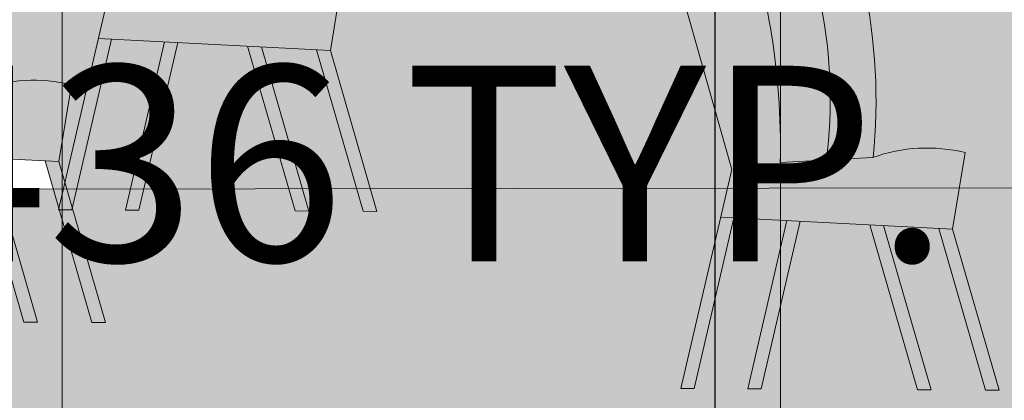
# Model space of a CAD drawing. Units: millimetres. Extents: x 11032 to 26788, y 3406 to 24505.
# Tile 7 of 78: x 15812 to 16566, y 7421 to 7713. Entities that reach past the tile are written whole.
import ezdxf

# ---------------------------------------------------------------- set-up
doc = ezdxf.new("R2010")
doc.units = ezdxf.units.MM
doc.header["$MEASUREMENT"] = 0
for name, color, linetype, lineweight in [('A-ANNO-DIMS', 2, 'Continuous', 18), ('A-FURN', 8, 'Continuous', 13), ('A-FURN-PATT', 8, 'Continuous', 13), ('A-GLAZ', 250, 'Continuous', 20), ('A-WALL-INTR', 8, 'Continuous', 18)]:
    doc.layers.add(name, color=color, linetype=linetype, lineweight=lineweight)
doc.layers.add('A-GLAZ-FRAM-PATT', color=250, linetype='Continuous', lineweight=13, true_color=0x262627)
doc.layers.add('A-WALL-INTR-PATT', color=251, linetype='Continuous', lineweight=13, true_color=0x6c6b6a)
doc.styles.get("Standard").update_dxf_attribs({"font": 'arial.ttf'})
doc.dimstyles.get("Standard").update_dxf_attribs({"dimtxt": 150, "dimasz": 100, "dimexe": 10, "dimexo": 5, "dimgap": 5, "dimtad": 0, "dimtih": 1, "dimtoh": 1, "dimdec": 0, "dimzin": 0, "dimdsep": 46, "dimtxsty": 'Standard', "dimcen": 0.09, "dimadec": 0, "dimazin": 0, "dimtfac": 1, "dimtdec": 0, "dimtofl": 0, "dimtmove": 0, "dimatfit": 3, "dimfxl": 1, "dimtolj": 1, "dimtzin": 0, "dimarcsym": 0})

# ---------------------------------------------------------------- blocks, each defined once
blk = doc.blocks.new('DINING-CHAIR-ELEV')
blk.add_line((228.68, 123.43), (51.04, 132.61))
for points in [[(0, 379.55), (49.45, 435.94), (114.12, 434.53)], [(61.18, 132.09), (30.79, 1.16), (20.53, 1.21), (59.55, 169.26), (0, 379.55), (61.9, 377.89)], [(111.9, 129.47), (82.06, 0.91), (71.8, 0.96), (101.76, 129.99)], [(165.28, 126.71), (201.76, 0.31), (212.19, 0.26), (175.85, 126.16)]]:
    blk.add_lwpolyline(points)
for points in [[(218.11, 123.98), (253.88, 0.05), (264.3, 0), (228.68, 123.43), (238.32, 182.18, 0.148451), (167.47, 178.33), (96.61, 174.48, 0.097012), (61.9, 377.89), (114.12, 434.53, -0.154833), (167.82, 178.46)], [(132.04, 176.4, 0.156877), (88.01, 406.21), (24.72, 407.74)]]:
    blk.add_lwpolyline(points, format="xyb")
blk = doc.blocks.new('*D16')
at = {"layer": 'A-ANNO-DIMS', "color": 0, "lineweight": -2, "transparency": 16777216}
for p, q in [((15741.74, 7821.05), (15812.13, 7821.05)), ((15802.13, 7721.05), (15802.13, 7685.69)), ((15802.13, 7485.11), (15802.13, 7520.47)), ((15741.74, 7385.11), (15812.13, 7385.11))]:
    blk.add_line(p, q, dxfattribs=at)
at = {"layer": 'A-ANNO-DIMS', "color": 0, "transparency": 16777216}
for points in [[(15785.47, 7721.05), (15818.8, 7721.05), (15802.13, 7821.05)], [(15785.47, 7485.11), (15818.8, 7485.11), (15802.13, 7385.11)]]:
    blk.add_solid(points, dxfattribs=at)
at = {"layer": 'Defpoints', "color": 0, "transparency": 16777216}
for p in [(15736.74, 7821.05), (15802.13, 7821.05), (15736.74, 7385.11)]:
    blk.add_point(p, dxfattribs=at)
at = {"layer": 'A-ANNO-DIMS', "color": 0, "transparency": 16777216, "insert": (15802.13, 7603.08), "char_height": 150, "attachment_point": 5}
blk.add_mtext('\\A1;CHAIR 436 TYP.', dxfattribs=at)
blk = doc.blocks.new('*D17')
at = {"layer": 'A-ANNO-DIMS', "color": 0, "lineweight": -2, "transparency": 16777216}
for p, q in [((15472.44, 7380.11), (15472.44, 7309.72)), ((15736.74, 7380.11), (15736.74, 7309.72)), ((15572.44, 7319.72), (15636.74, 7319.72)), ((15736.74, 7319.72), (15836.74, 7319.72))]:
    blk.add_line(p, q, dxfattribs=at)
at = {"layer": 'A-ANNO-DIMS', "color": 0, "transparency": 16777216}
for points in [[(15572.44, 7336.38), (15572.44, 7303.05), (15472.44, 7319.72)], [(15636.74, 7336.38), (15636.74, 7303.05), (15736.74, 7319.72)]]:
    blk.add_solid(points, dxfattribs=at)
at = {"layer": 'Defpoints', "color": 0, "transparency": 16777216}
for p in [(15472.44, 7385.11), (15736.74, 7385.11), (15736.74, 7319.72)]:
    blk.add_point(p, dxfattribs=at)
at = {"layer": 'A-ANNO-DIMS', "color": 0, "transparency": 16777216, "insert": (16266.37, 7319.72), "char_height": 150, "attachment_point": 5}
blk.add_mtext('\\A1;264 TYP.', dxfattribs=at)
blk = doc.blocks.new('*D36')
at = {"layer": 'A-ANNO-DIMS', "color": 0, "lineweight": -2, "transparency": 16777216}
for p, q in [((12301.26, 17115.89), (12301.26, 24416.86)), ((25397.4, 4466.4), (25397.4, 24416.86)), ((12401.26, 24406.86), (18569.2, 24406.86)), ((25297.4, 24406.86), (19129.47, 24406.86))]:
    blk.add_line(p, q, dxfattribs=at)
at = {"layer": 'A-ANNO-DIMS', "color": 0, "transparency": 16777216}
for points in [[(12401.26, 24423.52), (12401.26, 24390.19), (12301.26, 24406.86)], [(25297.4, 24423.52), (25297.4, 24390.19), (25397.4, 24406.86)]]:
    blk.add_solid(points, dxfattribs=at)
at = {"layer": 'Defpoints', "color": 0, "transparency": 16777216}
for p in [(25397.4, 24406.86), (12301.26, 17110.89), (25397.4, 4461.4)]:
    blk.add_point(p, dxfattribs=at)
at = {"layer": 'A-ANNO-DIMS', "color": 0, "transparency": 16777216, "insert": (18849.33, 24406.86), "char_height": 150, "attachment_point": 5}
blk.add_mtext('\\A1;13096', dxfattribs=at)
blk = doc.blocks.new('*D37')
at = {"layer": 'A-ANNO-DIMS', "color": 0, "lineweight": -2, "transparency": 16777216}
for p, q in [((18087.74, 23450.36), (11334.76, 23450.36)), ((11344.76, 23350.36), (11344.76, 14037.46)), ((11344.76, 4561.4), (11344.76, 13874.29)), ((12927.66, 4461.4), (11334.76, 4461.4))]:
    blk.add_line(p, q, dxfattribs=at)
at = {"layer": 'A-ANNO-DIMS', "color": 0, "transparency": 16777216}
for points in [[(11328.1, 23350.36), (11361.43, 23350.36), (11344.76, 23450.36)], [(11328.1, 4561.4), (11361.43, 4561.4), (11344.76, 4461.4)]]:
    blk.add_solid(points, dxfattribs=at)
at = {"layer": 'Defpoints', "color": 0, "transparency": 16777216}
for p in [(11344.76, 23450.36), (18092.74, 23450.36), (12932.66, 4461.4)]:
    blk.add_point(p, dxfattribs=at)
at = {"layer": 'A-ANNO-DIMS', "color": 0, "transparency": 16777216, "insert": (11344.76, 13955.88), "char_height": 150, "attachment_point": 5}
blk.add_mtext('\\A1;18989', dxfattribs=at)
blk = doc.blocks.new('*D49')
at = {"layer": 'A-ANNO-DIMS', "color": 0, "lineweight": -2, "transparency": 16777216}
for p, q in [((17953.45, 10206.41), (17953.45, 3494.9)), ((14996.4, 6406.4), (14996.4, 3494.9)), ((15096.4, 3504.9), (16244.67, 3504.9)), ((17853.45, 3504.9), (16705.18, 3504.9))]:
    blk.add_line(p, q, dxfattribs=at)
at = {"layer": 'A-ANNO-DIMS', "color": 0, "transparency": 16777216}
for points in [[(15096.4, 3521.57), (15096.4, 3488.23), (14996.4, 3504.9)], [(17853.45, 3521.57), (17853.45, 3488.23), (17953.45, 3504.9)]]:
    blk.add_solid(points, dxfattribs=at)
at = {"layer": 'Defpoints', "color": 0, "transparency": 16777216}
for p in [(17953.45, 10211.41), (14996.4, 6411.4), (17953.45, 3504.9)]:
    blk.add_point(p, dxfattribs=at)
at = {"layer": 'A-ANNO-DIMS', "color": 0, "transparency": 16777216, "insert": (16474.93, 3504.9), "char_height": 150, "attachment_point": 5}
blk.add_mtext('\\A1;2957', dxfattribs=at)
blk = doc.blocks.new('*D57')
at = {"layer": 'A-ANNO-DIMS', "color": 0, "lineweight": -2, "transparency": 16777216}
for p, q in [((14994.7, 7266.4), (14994.7, 24416.86)), ((20894.7, 7266.4), (20894.7, 24416.86)), ((15094.7, 24406.86), (17715.98, 24406.86)), ((20794.7, 24406.86), (18173.42, 24406.86))]:
    blk.add_line(p, q, dxfattribs=at)
at = {"layer": 'A-ANNO-DIMS', "color": 0, "transparency": 16777216}
for points in [[(15094.7, 24423.52), (15094.7, 24390.19), (14994.7, 24406.86)], [(20794.7, 24423.52), (20794.7, 24390.19), (20894.7, 24406.86)]]:
    blk.add_solid(points, dxfattribs=at)
at = {"layer": 'Defpoints', "color": 0, "transparency": 16777216}
for p in [(20894.7, 24406.86), (14994.7, 7261.4), (20894.7, 7261.4)]:
    blk.add_point(p, dxfattribs=at)
at = {"layer": 'A-ANNO-DIMS', "color": 0, "transparency": 16777216, "insert": (17944.7, 24406.86), "char_height": 150, "attachment_point": 5}
blk.add_mtext('\\A1;5900', dxfattribs=at)
blk = doc.blocks.new('*D60')
at = {"layer": 'A-ANNO-DIMS', "color": 0, "lineweight": -2, "transparency": 16777216}
for p, q in [((14994.7, 7266.4), (14994.7, 24416.86)), ((16344.7, 7266.4), (16344.7, 24416.86)), ((15094.7, 24406.86), (15448.04, 24406.86)), ((16244.7, 24406.86), (15891.36, 24406.86))]:
    blk.add_line(p, q, dxfattribs=at)
at = {"layer": 'A-ANNO-DIMS', "color": 0, "transparency": 16777216}
for points in [[(15094.7, 24423.52), (15094.7, 24390.19), (14994.7, 24406.86)], [(16244.7, 24423.52), (16244.7, 24390.19), (16344.7, 24406.86)]]:
    blk.add_solid(points, dxfattribs=at)
at = {"layer": 'Defpoints', "color": 0, "transparency": 16777216}
for p in [(16344.7, 24406.86), (14994.7, 7261.4), (16344.7, 7261.4)]:
    blk.add_point(p, dxfattribs=at)
at = {"layer": 'A-ANNO-DIMS', "color": 0, "transparency": 16777216, "insert": (15669.7, 24406.86), "char_height": 150, "attachment_point": 5}
blk.add_mtext('\\A1;1350', dxfattribs=at)
blk = doc.blocks.new('*D69')
at = {"layer": 'A-ANNO-DIMS', "color": 0, "lineweight": -2, "transparency": 16777216}
for p, q in [((13956.97, 9937.95), (14056.97, 9937.95)), ((14056.97, 9937.95), (15432.5, 8990.95)), ((17944.61, 7261.4), (17944.79, 7261.4)), ((17944.7, 7261.31), (17944.7, 7261.49))]:
    blk.add_line(p, q, dxfattribs=at)
at = {"layer": 'A-ANNO-DIMS', "color": 0, "transparency": 16777216}
blk.add_solid([(15441.95, 9004.68), (15423.05, 8977.22), (15514.87, 8934.24)], dxfattribs=at)
at = {"layer": 'Defpoints', "color": 0, "transparency": 16777216}
for p in [(15514.87, 8934.24), (17944.7, 7261.4)]:
    blk.add_point(p, dxfattribs=at)
at = {"layer": 'A-ANNO-DIMS', "color": 0, "transparency": 16777216, "insert": (13494.04, 9937.95), "char_height": 150, "attachment_point": 5}
blk.add_mtext('\\A1;2X R2950', dxfattribs=at)

msp = doc.modelspace()

# ---------------------------------------------------------------- hatches: boundary and pattern name
at = {"layer": 'A-FURN-PATT'}
h = msp.add_hatch(color=256, dxfattribs=at)
h.set_gradient(color1=(82, 15, 16), color2=(153, 0, 38), name='CURVED')
h.paths.add_polyline_path([(16952.125, 8119), (16926.017, 8147.32, 0.1568775), (16881.989, 7917.509), (16917.415, 7915.583, -0.0970121)], flags=0)
h.paths.add_polyline_path([(16899.908, 8175.64), (16964.58, 8177.046), (17014.03, 8120.657), (16954.484, 7910.365), (16972.017, 7834.84), (16977.75, 7834.965), (17027.199, 7778.576), (16967.653, 7568.284), (17006.665, 7400.238), (16996.411, 7400.187), (16966.016, 7531.114), (16925.439, 7529.018), (16955.395, 7399.983), (16945.141, 7399.932), (16915.295, 7528.494), (16861.916, 7525.736), (16825.435, 7399.337), (16815.012, 7399.285), (16851.35, 7525.19), (16809.087, 7523.007), (16773.319, 7399.078), (16762.896, 7399.026), (16798.521, 7522.461), (16788.882, 7581.207, -0.1476694), (16859.382, 7577.482, -0.1528132), (16911.41, 7830.579), (16902.125, 7870.575), (16848.746, 7867.817), (16830.506, 7804.617), (16830.506, 7793.515), (16827.302, 7793.515), (16812.265, 7741.418), (16801.842, 7741.366), (16816.893, 7793.515), (16775.261, 7793.515), (16760.15, 7741.159), (16749.727, 7741.107), (16764.853, 7793.515), (16650.704, 7793.515), (16662.994, 7750.932), (16652.571, 7750.983), (16640.296, 7793.515), (16598.663, 7793.515), (16610.879, 7751.191), (16600.455, 7751.242), (16588.255, 7793.515), (16490.425, 7793.515), (16480.749, 7751.837), (16470.495, 7751.888), (16480.159, 7793.515), (16443.833, 7793.515, -0.1094051), (16465.746, 7607.731, -0.1476694), (16536.246, 7611.456), (16526.606, 7552.71), (16562.232, 7429.275), (16551.809, 7429.327), (16516.041, 7553.255), (16473.778, 7555.439), (16510.116, 7429.534), (16499.693, 7429.586), (16463.212, 7555.985), (16409.833, 7558.743), (16379.987, 7430.181), (16369.733, 7430.232), (16394.704, 7537.793), (16394.704, 7559.524), (16359.112, 7561.363), (16328.717, 7430.435), (16318.463, 7430.486), (16344.704, 7543.521), (16344.704, 7643.635), (16302.264, 7793.515), (16205.738, 7793.515), (16227.021, 7719.773), (16216.598, 7719.825), (16195.329, 7793.515), (16153.697, 7793.515), (16174.905, 7720.032), (16164.482, 7720.084), (16143.289, 7793.515), (15844.423, 7793.515), (15844.423, 7804.617), (16140.084, 7804.617), (16128.001, 7846.483), (16191.395, 7843.208), (16201.035, 7901.954, 0.1484508), (16130.184, 7898.102), (16059.333, 7894.25, 0.0970121), (16024.622, 8097.666), (16076.839, 8154.307, -0.1548334), (16130.535, 7898.229, -0.1476694), (16201.035, 7901.954), (16191.395, 7843.208), (16202.533, 7804.617), (16299.12, 7804.617), (16297.929, 7808.825), (16347.378, 7865.214), (16412.05, 7863.808, -0.0295496), (16434.494, 7817.915), (16458.237, 7920.19), (16398.691, 8130.481), (16448.141, 8186.871), (16512.813, 8185.465, -0.1548334), (16566.508, 7929.387, -0.1476694), (16637.008, 7933.112), (16627.369, 7874.366), (16647.499, 7804.617), (16742.939, 7804.617), (16741.107, 8264.696), (17994.704, 8264.696), (17994.704, 7796.661), (18112.02, 7796.661), (18134.447, 7874.366), (18124.807, 7933.112, -0.1476694), (18195.307, 7929.387, -0.1548334), (18249.003, 8185.465), (18313.675, 8186.871), (18363.124, 8130.481), (18303.578, 7920.19), (18311.087, 7887.847, -0.0273017), (18332.016, 7930.161), (18396.688, 7931.567), (18446.137, 7875.177), (18423.905, 7796.661), (18470.25, 7796.661), (18470.25, 7785.559), (18420.761, 7785.559), (18386.591, 7664.886), (18425.604, 7496.839), (18415.35, 7496.788), (18384.955, 7627.716), (18344.377, 7625.62), (18374.333, 7496.584), (18364.079, 7496.533), (18334.233, 7625.095), (18280.854, 7622.338), (18244.373, 7495.938), (18233.95, 7495.887), (18270.288, 7621.792), (18228.026, 7619.608), (18192.257, 7495.679), (18181.834, 7495.628), (18217.46, 7619.062), (18207.82, 7677.808, -0.1476694), (18278.32, 7674.083, -0.0514181), (18278.516, 7762.821), (18273.237, 7785.559), (18171.265, 7785.559), (18161.36, 7751.242), (18150.937, 7751.191), (18160.856, 7785.559), (18119.224, 7785.559), (18109.244, 7750.983), (18098.821, 7750.932), (18108.815, 7785.559), (17852.794, 7785.559), (17866.18, 7739.181), (17855.756, 7739.233), (17842.386, 7785.559), (17800.753, 7785.559), (17814.064, 7739.44), (17803.641, 7739.492), (17790.345, 7785.559), (17694.491, 7785.559), (17685.986, 7748.922, -0.0882745), (17728.687, 7746.171), (17719.047, 7687.425), (17754.673, 7563.99), (17744.25, 7564.042), (17708.482, 7687.971), (17666.219, 7690.154), (17702.557, 7564.249), (17692.134, 7564.301), (17655.653, 7690.7), (17602.274, 7693.458), (17572.428, 7564.896), (17562.174, 7564.947), (17592.13, 7693.982), (17551.553, 7696.078), (17521.158, 7565.151), (17510.903, 7565.202), (17549.916, 7733.248), (17535.103, 7785.559), (17484.167, 7785.559), (17484.167, 7796.661), (17531.96, 7796.661), (17490.37, 7943.54), (17539.819, 7999.929), (17604.491, 7998.523, -0.0802486), (17652.289, 7869.096), (17661.422, 7908.439), (17601.876, 8118.731), (17651.326, 8175.12), (17715.998, 8173.714, -0.1548334), (17769.694, 7917.637, -0.1476694), (17840.194, 7921.361), (17830.554, 7862.615), (17849.59, 7796.661), (17894.704, 7796.661), (17894.704, 8239.696), (16741.207, 8239.696), (16742.939, 7804.617), (16768.057, 7804.617), (16785.352, 7864.542), (16775.713, 7923.288, -0.1476694), (16846.212, 7919.563, -0.1548334)], flags=17)
h.paths.add_polyline_path([(16899.908, 8175.64), (16964.58, 8177.046), (17014.03, 8120.657), (16954.484, 7910.365), (16993.496, 7742.318), (16983.242, 7742.267), (16952.847, 7873.195), (16912.27, 7871.099), (16942.225, 7742.064), (16931.971, 7742.013), (16902.125, 7870.575), (16848.746, 7867.817), (16812.265, 7741.418), (16801.842, 7741.366), (16838.181, 7867.271), (16795.918, 7865.087), (16760.15, 7741.159), (16749.727, 7741.107), (16785.352, 7864.542), (16775.713, 7923.288, -0.1476694), (16846.212, 7919.563, -0.1548334)], flags=0)
h.paths.add_polyline_path([(16899.908, 8175.64), (16964.58, 8177.046), (17014.03, 8120.657), (16954.484, 7910.365), (16972.017, 7834.84), (16977.75, 7834.965), (17027.199, 7778.576), (16967.653, 7568.284), (17006.665, 7400.238), (16996.411, 7400.187), (16966.016, 7531.114), (16925.439, 7529.018), (16955.395, 7399.983), (16945.141, 7399.932), (16915.295, 7528.494), (16861.916, 7525.736), (16825.435, 7399.337), (16815.012, 7399.285), (16851.35, 7525.19), (16809.087, 7523.007), (16773.319, 7399.078), (16762.896, 7399.026), (16798.521, 7522.461), (16788.882, 7581.207, -0.1476694), (16859.382, 7577.482, -0.1528132), (16911.41, 7830.579), (16902.125, 7870.575), (16848.746, 7867.817), (16830.506, 7804.617), (16830.506, 7793.515), (16827.302, 7793.515), (16812.265, 7741.418), (16801.842, 7741.366), (16816.893, 7793.515), (16775.261, 7793.515), (16760.15, 7741.159), (16749.727, 7741.107), (16764.853, 7793.515), (16650.704, 7793.515), (16662.994, 7750.932), (16652.571, 7750.983), (16640.296, 7793.515), (16598.663, 7793.515), (16610.879, 7751.191), (16600.455, 7751.242), (16588.255, 7793.515), (16490.425, 7793.515), (16480.749, 7751.837), (16470.495, 7751.888), (16480.159, 7793.515), (16443.833, 7793.515, -0.1094051), (16465.746, 7607.731, -0.1476694), (16536.246, 7611.456), (16526.606, 7552.71), (16562.232, 7429.275), (16551.809, 7429.327), (16516.041, 7553.255), (16473.778, 7555.439), (16510.116, 7429.534), (16499.693, 7429.586), (16463.212, 7555.985), (16409.833, 7558.743), (16379.987, 7430.181), (16369.733, 7430.232), (16394.704, 7537.793), (16394.704, 7559.524), (16359.112, 7561.363), (16328.717, 7430.435), (16318.463, 7430.486), (16344.704, 7543.521), (16344.704, 7643.635), (16302.264, 7793.515), (16205.738, 7793.515), (16227.021, 7719.773), (16216.598, 7719.825), (16195.329, 7793.515), (16153.697, 7793.515), (16174.905, 7720.032), (16164.482, 7720.084), (16143.289, 7793.515), (15844.423, 7793.515), (15844.423, 7804.617), (16140.084, 7804.617), (16128.001, 7846.483), (16191.395, 7843.208), (16201.035, 7901.954, 0.1484508), (16130.184, 7898.102), (16059.333, 7894.25, 0.0970121), (16024.622, 8097.666), (16076.839, 8154.307, -0.1548334), (16130.535, 7898.229, -0.1476694), (16201.035, 7901.954), (16191.395, 7843.208), (16202.533, 7804.617), (16299.12, 7804.617), (16297.929, 7808.825), (16347.378, 7865.214), (16412.05, 7863.808, -0.0295496), (16434.494, 7817.915), (16458.237, 7920.19), (16398.691, 8130.481), (16448.141, 8186.871), (16512.813, 8185.465, -0.1548334), (16566.508, 7929.387, -0.1476694), (16637.008, 7933.112), (16627.369, 7874.366), (16647.499, 7804.617), (16742.939, 7804.617), (16741.207, 8239.696), (16741.107, 8264.696), (17994.704, 8264.696), (17994.704, 7796.661), (18112.02, 7796.661), (18134.447, 7874.366), (18124.807, 7933.112, -0.1476694), (18195.307, 7929.387, -0.1548334), (18249.003, 8185.465), (18313.675, 8186.871), (18363.124, 8130.481), (18303.578, 7920.19), (18311.087, 7887.847, -0.0273017), (18332.016, 7930.161), (18396.688, 7931.567), (18446.137, 7875.177), (18423.905, 7796.661), (18470.25, 7796.661), (18470.25, 7785.559), (18420.761, 7785.559), (18386.591, 7664.886), (18425.604, 7496.839), (18415.35, 7496.788), (18384.955, 7627.716), (18344.377, 7625.62), (18374.333, 7496.584), (18364.079, 7496.533), (18334.233, 7625.095), (18280.854, 7622.338), (18244.373, 7495.938), (18233.95, 7495.887), (18270.288, 7621.792), (18228.026, 7619.608), (18192.257, 7495.679), (18181.834, 7495.628), (18217.46, 7619.062), (18207.82, 7677.808, -0.1476694), (18278.32, 7674.083, -0.0514181), (18278.516, 7762.821), (18273.237, 7785.559), (18171.265, 7785.559), (18161.36, 7751.242), (18150.937, 7751.191), (18160.856, 7785.559), (18119.224, 7785.559), (18109.244, 7750.983), (18098.821, 7750.932), (18108.815, 7785.559), (17852.794, 7785.559), (17866.18, 7739.181), (17855.756, 7739.233), (17842.386, 7785.559), (17800.753, 7785.559), (17814.064, 7739.44), (17803.641, 7739.492), (17790.345, 7785.559), (17694.491, 7785.559), (17685.986, 7748.922, -0.0882745), (17728.687, 7746.171), (17719.047, 7687.425), (17754.673, 7563.99), (17744.25, 7564.042), (17708.482, 7687.971), (17666.219, 7690.154), (17702.557, 7564.249), (17692.134, 7564.301), (17655.653, 7690.7), (17602.274, 7693.458), (17572.428, 7564.896), (17562.174, 7564.947), (17592.13, 7693.982), (17551.553, 7696.078), (17521.158, 7565.151), (17510.903, 7565.202), (17549.916, 7733.248), (17535.103, 7785.559), (17484.167, 7785.559), (17484.167, 7796.661), (17531.96, 7796.661), (17490.37, 7943.54), (17539.819, 7999.929), (17604.491, 7998.523, -0.0802486), (17652.289, 7869.096), (17661.422, 7908.439), (17601.876, 8118.731), (17651.326, 8175.12), (17715.998, 8173.714, -0.1548334), (17769.694, 7917.637, -0.1476694), (17840.194, 7921.361), (17830.554, 7862.615), (17849.59, 7796.661), (17894.704, 7796.661), (17894.704, 8239.696), (16741.207, 8239.696), (16742.939, 7804.617), (16768.057, 7804.617), (16785.352, 7864.542), (16775.713, 7923.288, -0.1476694), (16846.212, 7919.563, -0.1548334)], flags=17)
h = msp.add_hatch(color=256, dxfattribs=at)
h.set_gradient(color1=(153, 27, 30), color2=(153, 38, 0), name='SPHERICAL')
h.paths.add_polyline_path([(15534.344, 7763), (15472.44, 7764.657), (15531.986, 7554.365), (15523.479, 7517.719), (15640.736, 7511.661), (15653.713, 7567.556, 0.0295203), (15639.906, 7563.436), (15569.055, 7559.583, 0.0970121)], flags=16)
h.paths.add_polyline_path([(15560.453, 7791.32), (15534.344, 7763, -0.0970121), (15569.055, 7559.583), (15604.48, 7561.509, 0.1568775)], flags=16)
h.paths.add_polyline_path([(15586.562, 7819.64), (15560.453, 7791.32, -0.1568775), (15604.48, 7561.509), (15640.246, 7563.454, 0.154898)], flags=17)
h.paths.add_polyline_path([(15560.453, 7791.32), (15497.165, 7792.851), (15472.44, 7764.657), (15534.344, 7763)], flags=16)
h.paths.add_polyline_path([(15586.562, 7819.64), (15521.889, 7821.046), (15497.165, 7792.851), (15560.453, 7791.32)], flags=17)
h.paths.add_polyline_path([(15790.874, 7662.689, 0.021469), (15780.879, 7659.53), (15710.028, 7655.677, 0.0970121), (15675.317, 7859.094), (15665.772, 7859.35), (15665.799, 7675.745), (15672.959, 7650.459), (15665.807, 7619.654), (15665.808, 7613.744), (15790.755, 7607.288)], flags=17)
h.paths.add_polyline_path([(15665.772, 7859.35), (15613.413, 7860.751), (15665.799, 7675.745)], flags=16)
h.paths.add_polyline_path([(15701.426, 7887.414), (15665.767, 7888.277), (15665.772, 7859.35), (15675.317, 7859.094)], flags=16)
h.paths.add_polyline_path([(15727.534, 7915.735), (15665.763, 7917.077), (15665.767, 7888.277), (15701.426, 7887.414)], flags=17)
h.paths.add_polyline_path([(15665.763, 7917.077), (15662.862, 7917.14), (15638.137, 7888.946), (15665.767, 7888.277)], flags=17)
h.paths.add_polyline_path([(15665.767, 7888.277), (15638.137, 7888.946), (15613.413, 7860.751), (15665.772, 7859.35)], flags=16)
h.paths.add_polyline_path([(15701.426, 7887.414), (15675.317, 7859.094, -0.0970121), (15710.028, 7655.677), (15745.453, 7657.604, 0.1568775)], flags=16)
h.paths.add_polyline_path([(15844.495, 7664.925), (15844.384, 7864.461), (15821.312, 7945.94), (15870.762, 8002.329), (15935.434, 8000.923, -0.1195917), (15991.005, 7804.617), (16002.667, 7804.617), (16022.264, 7889.032), (15962.718, 8099.323), (16024.622, 8097.666), (16076.839, 8154.307, -0.1548334), (16130.535, 7898.229, -0.1476694), (16201.035, 7901.954), (16191.395, 7843.208), (16202.533, 7804.617), (16299.12, 7804.617), (16297.929, 7808.825), (16347.378, 7865.214), (16412.05, 7863.808, -0.0295496), (16434.494, 7817.915), (16458.237, 7920.19), (16398.691, 8130.481), (16460.595, 8128.825), (16512.813, 8185.465, -0.1548334), (16566.508, 7929.387, -0.1476694), (16637.008, 7933.112), (16627.369, 7874.366), (16647.499, 7804.617), (16830.506, 7804.617), (16830.506, 7793.515), (16650.704, 7793.515), (16662.994, 7750.932), (16652.571, 7750.983), (16640.296, 7793.515), (16490.425, 7793.515), (16480.749, 7751.837), (16470.495, 7751.888), (16480.159, 7793.515), (16443.833, 7793.515, -0.1094051), (16465.746, 7607.731, -0.1476694), (16536.246, 7611.456), (16526.606, 7552.71), (16562.232, 7429.275), (16551.809, 7429.327), (16516.041, 7553.255), (16473.778, 7555.439), (16510.116, 7429.534), (16499.693, 7429.586), (16463.212, 7555.985), (16409.833, 7558.743), (16379.987, 7430.181), (16369.733, 7430.232), (16394.704, 7537.793), (16394.704, 7559.524), (16359.112, 7561.363), (16328.717, 7430.435), (16318.463, 7430.486), (16344.704, 7543.521), (16344.704, 7643.635), (16302.264, 7793.515), (16205.738, 7793.515), (16227.021, 7719.773), (16216.598, 7719.825), (16195.329, 7793.515), (16153.697, 7793.515), (16174.905, 7720.032), (16164.482, 7720.084), (16143.289, 7793.515), (16061.685, 7793.515), (16051.641, 7750.248, -0.0167144), (16059.629, 7748.571), (16049.99, 7689.825), (16085.615, 7566.39), (16075.192, 7566.442), (16039.424, 7690.371), (15997.161, 7692.554), (16033.5, 7566.649), (16023.077, 7566.701), (15986.595, 7693.1), (15933.216, 7695.858), (15903.371, 7567.296), (15893.116, 7567.347), (15923.072, 7696.382), (15882.495, 7698.478), (15852.409, 7568.882), (15877.716, 7481.201), (15867.293, 7481.253), (15842.372, 7567.599), (15841.846, 7567.602), (15842.08, 7568.609), (15831.524, 7605.182), (15790.755, 7607.288), (15790.744, 7602.228), (15825.6, 7481.46), (15815.177, 7481.512), (15778.696, 7607.911), (15725.317, 7610.669), (15701.389, 7507.6), (15736.743, 7385.107), (15726.32, 7385.159), (15696.749, 7487.614), (15695.471, 7482.107), (15685.217, 7482.158), (15691.06, 7507.327), (15690.552, 7509.088), (15650.881, 7511.137), (15649.743, 7506.234), (15684.627, 7385.366), (15674.204, 7385.418), (15645.103, 7486.248), (15644.2, 7482.362), (15633.946, 7482.413), (15639.413, 7505.961), (15637.723, 7511.817), (15584.344, 7514.575), (15554.498, 7386.013), (15544.244, 7386.064), (15574.2, 7515.099), (15533.623, 7517.195), (15503.228, 7386.268), (15492.974, 7386.319), (15531.986, 7554.365), (15472.44, 7764.657), (15497.165, 7792.851), (15521.889, 7821.046), (15586.562, 7819.64, -0.1548334), (15640.257, 7563.563, -0.0287549), (15653.713, 7567.556), (15665.807, 7619.654), (15665.799, 7675.745), (15613.413, 7860.751), (15638.137, 7888.946), (15662.862, 7917.14), (15665.763, 7917.077), (15727.534, 7915.735, -0.1548334), (15781.23, 7659.657, -0.1322263)])
h = msp.add_hatch(color=256, dxfattribs=at)
h.set_gradient(color1=(153, 27, 30), color2=(153, 38, 0), name='SPHERICAL')
h.paths.add_polyline_path([(15710.028, 7655.677), (15745.453, 7657.604, 0.1568775), (15701.426, 7887.414), (15675.317, 7859.094, -0.0970121)], flags=16)
h.paths.add_polyline_path([(15790.755, 7607.288), (15790.874, 7662.689, 0.021469), (15780.879, 7659.53), (15710.028, 7655.677, 0.0970121), (15675.317, 7859.094), (15665.772, 7859.35), (15665.799, 7675.745), (15672.959, 7650.459), (15665.807, 7619.654), (15665.808, 7613.744)], flags=17)
h.paths.add_polyline_path([(15653.713, 7567.556), (15665.807, 7619.654), (15665.799, 7675.745), (15613.413, 7860.751), (15662.862, 7917.14), (15727.534, 7915.735, -0.1548334), (15781.23, 7659.657, -0.1322263), (15844.495, 7664.925), (15844.384, 7864.461), (15821.312, 7945.94), (15883.216, 7944.283), (15935.434, 8000.923, -0.1195917), (15991.005, 7804.617), (16002.667, 7804.617), (16022.264, 7889.032), (15962.718, 8099.323), (16024.622, 8097.666), (16076.839, 8154.307, -0.1548334), (16130.535, 7898.229, -0.1476694), (16201.035, 7901.954), (16191.395, 7843.208), (16202.533, 7804.617), (16830.506, 7804.617), (16830.506, 7793.515), (16205.738, 7793.515), (16227.021, 7719.773), (16216.598, 7719.825), (16195.329, 7793.515), (16153.697, 7793.515), (16174.905, 7720.032), (16164.482, 7720.084), (16143.289, 7793.515), (16061.685, 7793.515), (16051.641, 7750.248, -0.0167144), (16059.629, 7748.571), (16049.99, 7689.825), (16085.615, 7566.39), (16075.192, 7566.442), (16039.424, 7690.371), (15997.161, 7692.554), (16033.5, 7566.649), (16023.077, 7566.701), (15986.595, 7693.1), (15933.216, 7695.858), (15903.371, 7567.296), (15893.116, 7567.347), (15923.072, 7696.382), (15882.495, 7698.478), (15852.409, 7568.882), (15877.716, 7481.201), (15867.293, 7481.253), (15842.372, 7567.599), (15841.846, 7567.602), (15842.08, 7568.609), (15831.524, 7605.182), (15790.755, 7607.288), (15790.744, 7602.228), (15825.6, 7481.46), (15815.177, 7481.512), (15778.696, 7607.911), (15725.317, 7610.669), (15701.389, 7507.6), (15736.743, 7385.107), (15726.32, 7385.159), (15696.749, 7487.614), (15695.471, 7482.107), (15685.217, 7482.158), (15705.262, 7568.502, 0.0841685), (15664.448, 7569.579), (15644.2, 7482.362), (15633.946, 7482.413), (15653.713, 7567.556, 0.0295203), (15639.906, 7563.436), (15569.055, 7559.583, 0.0970121), (15534.344, 7763), (15472.44, 7764.657), (15521.889, 7821.046), (15586.562, 7819.64, -0.1548334), (15640.257, 7563.563, -0.0287549)])
at = {"layer": 'A-GLAZ-FRAM-PATT'}
h = msp.add_hatch(color=256, dxfattribs=at)
h.paths.add_polyline_path([(17944.704, 7311.399), (16344.704, 7311.399), (16344.704, 7261.399), (17944.704, 7261.399)], flags=17)
h.paths.add_polyline_path([(16344.704, 7311.399), (15045.135, 7311.399, -0.9829047), (20844.273, 7311.399), (19544.704, 7311.399), (19544.704, 7261.399), (20894.704, 7261.399, 0.5148441), (16985.951, 10051.255, 0.3202679), (14994.704, 7261.399), (16344.704, 7261.399)])
h.paths.add_polyline_path([(18744.704, 7311.399), (17944.704, 7311.399), (17944.704, 7261.399), (18744.704, 7261.399)], flags=17)
h.paths.add_polyline_path([(19544.704, 7311.399), (18744.704, 7311.399), (18744.704, 7261.399), (19544.704, 7261.399)], flags=17)
h.paths.add_polyline_path([(18694.704, 7361.399), (17994.704, 7361.399), (17994.704, 7311.399), (18694.704, 7311.399)], flags=17)
h.paths.add_polyline_path([(18744.704, 7361.399), (18694.704, 7361.399), (18694.704, 7311.399), (18744.704, 7311.399)], flags=17)
h.paths.add_polyline_path([(17194.704, 7361.399), (17144.704, 7361.399), (17144.704, 7311.399), (17194.704, 7311.399)], flags=17)
h.paths.add_polyline_path([(17431.432, 7361.399), (17194.704, 7361.399), (17194.704, 7311.399), (17431.699, 7311.399)], flags=17)
h.paths.add_polyline_path([(17894.704, 7361.399), (17431.432, 7361.399), (17431.699, 7311.399), (17894.704, 7311.399)], flags=17)
h.paths.add_polyline_path([(17944.704, 7361.399), (17894.704, 7361.399), (17894.704, 7311.399), (17944.704, 7311.399)], flags=17)
h.paths.add_polyline_path([(17994.704, 7361.399), (17944.704, 7361.399), (17944.704, 7311.399), (17994.704, 7311.399)], flags=17)
h = msp.add_hatch(color=256, dxfattribs=at)
h.paths.add_polyline_path([(16734.609, 9896.863, 0.0333754), (16394.704, 9712.419), (16394.704, 7804.617), (16431.407, 7804.617), (16458.237, 7920.19), (16398.691, 8130.481), (16448.141, 8186.871), (16512.813, 8185.465, -0.1548334), (16566.508, 7929.387, -0.1476694), (16637.008, 7933.112), (16627.369, 7874.366), (16647.499, 7804.617), (16742.939, 7804.617)])
h.paths.add_polyline_path([(17094.704, 9961.399), (16886.403, 9961.399, 0.0142221), (16734.609, 9896.863), (16741.107, 8264.696), (17094.704, 8264.696)])
h.paths.add_polyline_path([(17417.202, 10027.292), (17194.704, 10011.399), (17194.704, 8264.696), (17426.61, 8264.696)])
h.paths.add_polyline_path([(17144.704, 8239.696), (17094.704, 8239.696), (17094.704, 7361.399), (16394.704, 7361.399), (16394.704, 7493.572), (16379.987, 7430.181), (16369.733, 7430.232), (16394.704, 7537.793), (16394.704, 7559.524), (16359.112, 7561.363), (16344.704, 7499.3), (16344.704, 7311.399), (17144.704, 7311.399)])
h.paths.add_polyline_path([(17194.704, 8239.696), (17144.704, 8239.696), (17144.704, 7361.399), (17194.704, 7361.399)])
at = {"layer": 'A-WALL-INTR-PATT'}
msp.add_hatch(color=256, dxfattribs=at).paths.add_polyline_path([(15843.607, 9260.247, 0.0062633), (15794.195, 9206.987), (15790.874, 7662.689, -0.1112179), (15844.495, 7664.925), (15844.384, 7864.461), (15821.312, 7945.94), (15844.324, 7972.181)])
h = msp.add_hatch(color=256, dxfattribs=at)
h.paths.add_polyline_path([(15302.659, 8457.059, 0.0281002), (15185.248, 8153.253), (15233.282, 7717.599), (15314.374, 7311.399), (15467.334, 7311.399), (15381.661, 7740.545)])
h.paths.add_polyline_path([(16344.704, 7543.521), (16344.704, 7643.635), (16302.264, 7793.515), (16205.738, 7793.515), (16227.021, 7719.773), (16216.598, 7719.825), (16195.329, 7793.515), (16153.697, 7793.515), (16174.905, 7720.032), (16164.482, 7720.084), (16143.289, 7793.515), (16061.685, 7793.515), (16051.641, 7750.248, -0.0167144), (16059.629, 7748.571), (16049.99, 7689.825), (16085.615, 7566.39), (16075.192, 7566.442), (16039.424, 7690.371), (15997.161, 7692.554), (16033.5, 7566.649), (16023.077, 7566.701), (15986.595, 7693.1), (15933.216, 7695.858), (15903.371, 7567.296), (15893.116, 7567.347), (15923.072, 7696.382), (15882.495, 7698.478), (15852.409, 7568.882), (15877.716, 7481.201), (15867.293, 7481.253), (15844.553, 7560.041), (15844.691, 7311.399), (16344.704, 7311.399), (16344.704, 7499.3), (16328.717, 7430.435), (16318.463, 7430.486)])
h.paths.add_polyline_path([(16742.983, 7793.515), (16650.704, 7793.515), (16662.994, 7750.932), (16652.571, 7750.983), (16640.296, 7793.515), (16598.663, 7793.515), (16610.879, 7751.191), (16600.455, 7751.242), (16588.255, 7793.515), (16490.425, 7793.515), (16480.749, 7751.837), (16470.495, 7751.888), (16480.159, 7793.515), (16443.833, 7793.515, -0.1094051), (16465.746, 7607.731, -0.1476694), (16536.246, 7611.456), (16526.606, 7552.71), (16562.232, 7429.275), (16551.809, 7429.327), (16516.041, 7553.255), (16473.778, 7555.439), (16510.116, 7429.534), (16499.693, 7429.586), (16463.212, 7555.985), (16409.833, 7558.743), (16394.704, 7493.572), (16394.704, 7361.399), (16744.704, 7361.399)])
h.paths.add_polyline_path([(17094.704, 8239.696), (16741.207, 8239.696), (16742.939, 7804.617), (16768.057, 7804.617), (16785.352, 7864.542), (16775.713, 7923.288, -0.1476694), (16846.212, 7919.563, -0.1548334), (16899.908, 8175.64), (16964.58, 8177.046), (17014.03, 8120.657), (16954.484, 7910.365), (16972.017, 7834.84), (16977.75, 7834.965), (17027.199, 7778.576), (16967.653, 7568.284), (17006.665, 7400.238), (16996.411, 7400.187), (16966.016, 7531.114), (16925.439, 7529.018), (16955.395, 7399.983), (16945.141, 7399.932), (16915.295, 7528.494), (16861.916, 7525.736), (16825.435, 7399.337), (16815.012, 7399.285), (16851.35, 7525.19), (16809.087, 7523.007), (16773.319, 7399.078), (16762.896, 7399.026), (16798.521, 7522.461), (16788.882, 7581.207, -0.1476694), (16859.382, 7577.482, -0.1528132), (16911.41, 7830.579), (16902.125, 7870.575), (16848.746, 7867.817), (16830.506, 7804.617), (16830.506, 7793.515), (16827.302, 7793.515), (16812.265, 7741.418), (16801.842, 7741.366), (16816.893, 7793.515), (16775.261, 7793.515), (16760.15, 7741.159), (16749.727, 7741.107), (16764.853, 7793.515), (16742.983, 7793.515), (16744.704, 7361.399), (17094.704, 7361.399)])
h.paths.add_polyline_path([(18950.929, 7931.023), (19015.601, 7932.429), (19065.05, 7876.04), (19005.504, 7665.748), (19014.012, 7629.102, -0.129191), (19069.892, 7841.762), (19134.564, 7843.167), (19168.958, 7803.946), (19202.145, 7841.791), (19246.92, 7840.817), (19212.932, 7960.847), (19262.382, 8017.236), (19327.054, 8015.831, -0.134919), (19382.824, 7793.43), (19562.845, 7793.43, -0.1257757), (19618.686, 8000.275), (19683.358, 8001.68), (19732.808, 7945.291), (19689.807, 7793.43), (19753.644, 7793.43, -0.0966843), (19805.964, 7950.707), (19870.637, 7952.112), (19920.086, 7895.723), (19891.121, 7793.43), (20039.255, 7793.43, -0.0897865), (20089.9, 7938.993), (20154.572, 7940.399), (20204.021, 7884.01), (20144.475, 7673.718), (20152.983, 7637.072, -0.1476694), (20223.483, 7633.347, -0.1548334), (20277.178, 7889.425), (20341.85, 7890.831), (20391.3, 7834.441), (20331.754, 7624.15), (20370.766, 7456.103), (20360.512, 7456.052), (20330.117, 7586.98), (20289.54, 7584.884), (20319.496, 7455.848), (20309.241, 7455.797), (20279.396, 7584.359), (20226.017, 7581.602), (20189.536, 7455.202), (20179.112, 7455.151), (20215.451, 7581.056), (20173.188, 7578.872), (20169.478, 7566.018), (20183.488, 7505.671), (20173.234, 7505.62), (20163.789, 7546.305), (20137.42, 7454.943), (20126.997, 7454.892), (20159.149, 7566.291), (20142.839, 7636.548), (20102.261, 7634.452), (20132.217, 7505.417), (20121.963, 7505.366), (20092.117, 7633.928), (20038.738, 7631.17), (20002.257, 7504.771), (19991.834, 7504.719), (20028.172, 7630.624), (19985.91, 7628.44), (19950.141, 7504.512), (19939.718, 7504.46), (19975.344, 7627.895), (19965.704, 7686.641, -0.1476694), (20036.204, 7682.916, -0.0576487), (20037.659, 7782.328), (19887.977, 7782.328), (19860.54, 7685.431), (19899.552, 7517.385), (19889.298, 7517.334), (19858.903, 7648.261), (19818.326, 7646.165), (19848.282, 7517.13), (19838.028, 7517.079), (19808.182, 7645.641), (19754.803, 7642.883), (19718.322, 7516.484), (19707.899, 7516.432), (19744.237, 7642.337), (19701.974, 7640.154), (19698.264, 7627.3), (19712.274, 7566.953), (19702.02, 7566.902), (19692.575, 7607.587), (19666.206, 7516.225), (19655.783, 7516.173), (19687.935, 7627.573), (19671.625, 7697.83), (19631.048, 7695.733), (19661.003, 7566.698), (19650.749, 7566.647), (19620.903, 7695.209), (19567.524, 7692.451), (19531.043, 7566.052), (19520.62, 7566), (19556.959, 7691.905), (19514.696, 7689.722), (19478.928, 7565.793), (19468.505, 7565.741), (19473, 7581.318), (19466.812, 7581.349), (19431.044, 7705.278), (19388.781, 7707.461), (19425.12, 7581.556), (19414.696, 7581.608), (19378.215, 7708.007), (19324.836, 7710.765), (19318.877, 7685.094, -0.0584523), (19320.513, 7584.307, -0.1476694), (19391.013, 7588.032), (19381.373, 7529.286), (19416.999, 7405.852), (19406.576, 7405.903), (19370.808, 7529.832), (19328.545, 7532.016), (19364.883, 7406.111), (19354.46, 7406.162), (19317.979, 7532.562), (19264.6, 7535.319), (19234.754, 7406.757), (19224.5, 7406.808), (19254.456, 7535.844), (19213.879, 7537.94), (19183.484, 7407.012), (19173.23, 7407.063), (19212.242, 7575.11), (19168.16, 7730.789), (19124.467, 7576.487), (19163.48, 7408.44), (19153.225, 7408.389), (19122.83, 7539.317), (19082.253, 7537.22), (19112.209, 7408.185), (19101.955, 7408.134), (19072.109, 7536.696), (19035.898, 7534.825), (19044.517, 7497.701), (19034.262, 7497.65), (19025.754, 7534.301), (19018.73, 7533.938), (18982.249, 7407.539), (18971.826, 7407.487), (19008.164, 7533.392), (18985.177, 7532.205), (18993.246, 7497.447), (18982.992, 7497.396), (18975.033, 7531.681), (18965.902, 7531.209), (18930.133, 7407.28), (18919.71, 7407.228), (18955.336, 7530.663), (18945.696, 7589.409, -0.0318483), (18960.996, 7592.142), (18953.146, 7625.958), (18899.767, 7623.2), (18863.286, 7496.801), (18852.863, 7496.749), (18889.201, 7622.654), (18846.938, 7620.47), (18811.17, 7496.542), (18800.747, 7496.49), (18836.373, 7619.924), (18826.733, 7678.67, -0.1476694), (18897.233, 7674.946, -0.1548334)], flags=16)
h = msp.add_hatch(color=256, dxfattribs=at)
h.set_gradient(color1=(254, 234, 185), color2=(254, 204, 102), name='CURVED')
h.paths.add_polyline_path([(15260.167, 7582.928), (15062.56, 7582.722, 0.023451), (15045.135, 7311.399), (15314.374, 7311.399)])
h.paths.add_polyline_path([(15413.095, 7583.087), (15260.167, 7582.928), (15314.374, 7311.399), (15467.334, 7311.399)])
h.paths.add_polyline_path([(15531.986, 7554.365), (15523.82, 7583.203), (15413.095, 7583.087), (15467.334, 7311.399), (15790.119, 7311.399), (15790.667, 7566.433), (15785.748, 7583.476), (15718.988, 7583.406), (15701.389, 7507.6), (15736.743, 7385.107), (15726.32, 7385.159), (15696.749, 7487.614), (15695.471, 7482.107), (15685.217, 7482.158), (15691.06, 7507.327), (15690.552, 7509.088), (15650.881, 7511.137), (15649.743, 7506.234), (15684.627, 7385.366), (15674.204, 7385.418), (15646.227, 7482.352), (15633.946, 7482.413), (15639.413, 7505.961), (15637.723, 7511.817), (15584.344, 7514.575), (15554.498, 7386.013), (15544.244, 7386.064), (15574.2, 7515.099), (15533.623, 7517.195), (15503.228, 7386.268), (15492.974, 7386.319)])
h.paths.add_polyline_path([(16344.704, 7499.3), (16328.717, 7430.435), (16318.463, 7430.486), (16344.704, 7543.521), (16344.704, 7584.059), (16080.595, 7583.783), (16085.615, 7566.39), (16075.192, 7566.442), (16070.19, 7583.773), (16028.57, 7583.729), (16033.5, 7566.649), (16023.077, 7566.701), (16018.165, 7583.718), (15907.156, 7583.603), (15903.371, 7567.296), (15893.116, 7567.347), (15896.888, 7583.592), (15855.814, 7583.549), (15852.409, 7568.882), (15877.716, 7481.201), (15867.293, 7481.253), (15844.553, 7560.041), (15844.691, 7311.399), (16344.704, 7311.399)])
h.paths.add_polyline_path([(15844.553, 7560.041), (15842.372, 7567.599), (15841.846, 7567.602), (15842.08, 7568.609), (15837.773, 7583.53), (15796.153, 7583.487), (15825.6, 7481.46), (15815.177, 7481.512), (15790.667, 7566.433), (15790.119, 7311.399), (15844.691, 7311.399)])
h.paths.add_polyline_path([(16394.704, 7493.572), (16379.987, 7430.181), (16369.733, 7430.232), (16394.704, 7537.793), (16394.704, 7559.524), (16359.112, 7561.363), (16344.704, 7499.3), (16344.704, 7311.399), (17144.704, 7311.399), (17144.704, 7584.893), (17094.704, 7584.841), (17094.704, 7361.399), (16394.704, 7361.399)])
h.paths.add_polyline_path([(17430.237, 7585.191), (17194.704, 7584.945), (17194.704, 7361.399), (17431.432, 7361.399)])
h.paths.add_polyline_path([(17894.704, 7585.675), (17748.458, 7585.522), (17754.673, 7563.99), (17744.25, 7564.042), (17738.053, 7585.511), (17696.433, 7585.468), (17702.557, 7564.249), (17692.134, 7564.301), (17686.028, 7585.457), (17577.175, 7585.344), (17572.428, 7564.896), (17562.174, 7564.947), (17566.907, 7585.333), (17525.833, 7585.29), (17521.158, 7565.151), (17510.903, 7565.202), (17515.565, 7585.28), (17430.237, 7585.191), (17431.432, 7361.399), (17894.704, 7361.399)])
h.paths.add_polyline_path([(18694.704, 7586.509), (18404.857, 7586.207), (18425.604, 7496.839), (18415.35, 7496.788), (18394.593, 7586.196), (18353.54, 7586.153), (18374.333, 7496.584), (18364.079, 7496.533), (18343.276, 7586.142), (18270.386, 7586.066), (18244.373, 7495.938), (18233.95, 7495.887), (18259.974, 7586.056), (18218.329, 7586.012), (18192.257, 7495.679), (18181.834, 7495.628), (18207.918, 7586.001), (17994.704, 7585.779), (17994.704, 7361.399), (18694.704, 7361.399)])
h.paths.add_polyline_path([(19317.979, 7532.562), (19264.6, 7535.319), (19234.754, 7406.757), (19224.5, 7406.808), (19254.456, 7535.844), (19213.879, 7537.94), (19183.484, 7407.012), (19173.23, 7407.063), (19212.242, 7575.11), (19208.862, 7587.045), (19127.433, 7586.96), (19124.467, 7576.487), (19163.48, 7408.44), (19153.225, 7408.389), (19122.83, 7539.317), (19082.253, 7537.22), (19112.209, 7408.185), (19101.955, 7408.134), (19072.109, 7536.696), (19035.898, 7534.825), (19044.517, 7497.701), (19034.262, 7497.65), (19025.754, 7534.301), (19018.73, 7533.938), (18982.249, 7407.539), (18971.826, 7407.487), (19008.164, 7533.392), (18985.177, 7532.205), (18993.246, 7497.447), (18982.992, 7497.396), (18975.033, 7531.681), (18965.902, 7531.209), (18930.133, 7407.28), (18919.71, 7407.228), (18955.336, 7530.663), (18946.129, 7586.771), (18889.236, 7586.712), (18863.286, 7496.801), (18852.863, 7496.749), (18878.825, 7586.701), (18837.179, 7586.657), (18811.17, 7496.542), (18800.747, 7496.49), (18826.768, 7586.647), (18794.704, 7586.613), (18794.704, 7361.399), (19494.704, 7361.399), (19494.704, 7587.343), (19485.145, 7587.333), (19478.928, 7565.793), (19468.505, 7565.741), (19473, 7581.318), (19466.812, 7581.349), (19465.091, 7587.312), (19423.471, 7587.269), (19425.12, 7581.556), (19414.696, 7581.608), (19413.066, 7587.258), (19390.882, 7587.235), (19381.373, 7529.286), (19416.999, 7405.852), (19406.576, 7405.903), (19370.808, 7529.832), (19328.545, 7532.016), (19364.883, 7406.111), (19354.46, 7406.162)])
h.paths.add_polyline_path([(19990.261, 7587.86), (19974.192, 7587.843), (19950.141, 7504.512), (19939.718, 7504.46), (19963.781, 7587.832), (19883.217, 7587.748), (19899.552, 7517.385), (19889.298, 7517.334), (19872.954, 7587.737), (19831.9, 7587.695), (19848.282, 7517.13), (19838.028, 7517.079), (19821.637, 7587.684), (19738.846, 7587.598), (19718.322, 7516.484), (19707.899, 7516.432), (19728.435, 7587.587), (19707.489, 7587.565), (19712.274, 7566.953), (19702.02, 7566.902), (19697.225, 7587.554), (19686.79, 7587.543), (19666.206, 7516.225), (19655.783, 7516.173), (19676.379, 7587.532), (19656.172, 7587.511), (19661.003, 7566.698), (19650.749, 7566.647), (19645.908, 7587.501), (19544.704, 7587.395), (19544.704, 7311.399), (19990.261, 7311.399)])
h.paths.add_polyline_path([(20190.261, 7455.206), (20179.112, 7455.151), (20190.261, 7493.779), (20190.261, 7579.754), (20173.188, 7578.872), (20169.478, 7566.018), (20183.488, 7505.671), (20173.234, 7505.62), (20163.789, 7546.305), (20137.42, 7454.943), (20126.997, 7454.892), (20159.149, 7566.291), (20154.102, 7588.03), (20113.048, 7587.988), (20132.217, 7505.417), (20121.963, 7505.366), (20102.785, 7587.977), (20026.249, 7587.897), (20002.257, 7504.771), (19990.261, 7504.711), (19990.261, 7311.399), (20190.261, 7311.399)])
h.paths.add_polyline_path([(20340.261, 7543.283), (20330.117, 7586.98), (20289.54, 7584.884), (20319.496, 7455.848), (20309.241, 7455.797), (20279.396, 7584.359), (20226.017, 7581.602), (20190.261, 7457.717), (20190.261, 7311.399), (20340.261, 7311.399)])
h.paths.add_polyline_path([(20826.171, 7588.731), (20340.261, 7588.225), (20340.261, 7587.504), (20370.766, 7456.103), (20360.512, 7456.052), (20340.261, 7543.283), (20340.261, 7311.399), (20844.273, 7311.399, 0.0239726)])

# ---------------------------------------------------------------- linework, layer by layer
at = {"layer": 'A-GLAZ'}
for p, q in [((16394.704, 7361.399), (16394.704, 9712.419)), ((16344.704, 7261.399), (16344.704, 9680.076))]:
    msp.add_line(p, q, dxfattribs=at)
for radius, start, end in [(2900, 0.987907, 179.012093), (2950, 108.965621, 181.942602)]:
    msp.add_arc((17944.704, 7261.399), radius, start, end, dxfattribs=at)
at = {"layer": 'A-WALL-INTR'}
for p, q in [((15843.607, 9260.247), (15844.691, 7311.399)), ((15062.56, 7582.722), (20826.171, 7588.731))]:
    msp.add_line(p, q, dxfattribs=at)

# ---------------------------------------------------------------- block references
at = {"layer": 'A-FURN'}
for p in [(15821.312, 7566.39), (15613.413, 7481.201), (16297.929, 7429.275)]:
    msp.add_blockref('DINING-CHAIR-ELEV', p, dxfattribs=at)

# ---------------------------------------------------------------- dimensions: what is measured, and where the dimension line sits
at = {"layer": 'A-ANNO-DIMS'}
for base, p1, p2, picture, middle in [((25397.404, 24406.858), (12301.265, 17110.885), (25397.404, 4461.399), '*D36', (18849.334, 24406.858)), ((20894.704, 24406.858), (14994.704, 7261.399), (20894.704, 7261.399), '*D57', (17944.704, 24406.858)), ((16344.704, 24406.858), (14994.704, 7261.399), (16344.704, 7261.399), '*D60', (15669.704, 24406.858)), ((17953.455, 3504.899), (14996.399, 6411.399), (17953.455, 10211.41), '*D49', (16474.927, 3504.899))]:
    dim = msp.add_linear_dim(base=base, p1=p1, p2=p2, dimstyle='Standard', override={"dimdec": 0, "dimlfac": 1, "dimrnd": 0, "dimzin": 0, "dimdsep": 46, "dimlunit": 2}, dxfattribs=at)
    dim.commit()
    dim.dimension.update_dxf_attribs({"geometry": picture, "text_midpoint": middle})
dim = msp.add_linear_dim(base=(11344.765, 23450.358), p1=(12932.665, 4461.399), p2=(18092.739, 23450.358), angle=90, dimstyle='Standard', override={"dimdec": 0, "dimlfac": 1, "dimrnd": 0, "dimzin": 0, "dimdsep": 46, "dimlunit": 2}, dxfattribs=at)
dim.commit()
dim.dimension.update_dxf_attribs({"geometry": '*D37', "text_midpoint": (11344.765, 13955.879)})
dim = msp.add_radius_dim(center=(17944.704, 7261.399), mpoint=(15514.87, 8934.244), text='2X <>', dimstyle='Standard', override={"dimdec": 0, "dimlfac": 1, "dimrnd": 0, "dimzin": 0, "dimdsep": 46, "dimlunit": 2}, dxfattribs=at)
dim.commit()
dim.dimension.update_dxf_attribs({"geometry": '*D69', "text_midpoint": (13494.04, 9937.951), "dimtype": 164})
dim = msp.add_linear_dim(base=(15802.134, 7821.046), p1=(15736.743, 7385.107), p2=(15736.743, 7821.046), angle=90, text='CHAIR <> TYP.', dimstyle='Standard', override={"dimdec": 0, "dimlfac": 1, "dimrnd": 0, "dimzin": 0, "dimdsep": 46, "dimlunit": 2}, dxfattribs=at)
dim.commit()
dim.dimension.update_dxf_attribs({"geometry": '*D16', "text_midpoint": (15802.134, 7603.076)})
dim = msp.add_linear_dim(base=(15736.743, 7319.716), p1=(15472.44, 7385.107), p2=(15736.743, 7385.107), text='<> TYP.', dimstyle='Standard', override={"dimdec": 0, "dimlfac": 1, "dimrnd": 0, "dimzin": 0, "dimdsep": 46, "dimlunit": 2}, dxfattribs=at)
dim.commit()
dim.dimension.update_dxf_attribs({"geometry": '*D17', "text_midpoint": (16266.368, 7319.716)})

doc.saveas('drawing.dxf')
